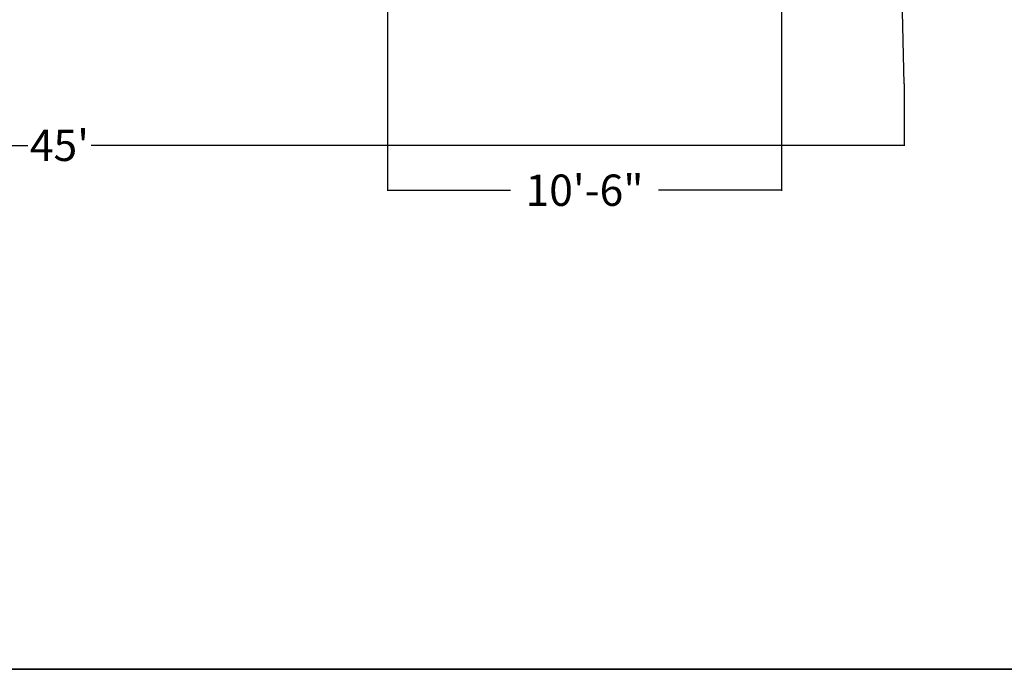
# Model space of a CAD drawing. Units: inches. Extents: x -269 to 4574, y -694 to 313.
# Tile 2 of 19: x 208 to 522, y -694 to -486. Entities that reach past the tile are written whole.
import ezdxf

# ---------------------------------------------------------------- set-up
doc = ezdxf.new("R2010")
doc.units = ezdxf.units.IN
doc.header["$MEASUREMENT"] = 0
for name, color, linetype, lineweight in [('BORDER', 7, 'Continuous', 35), ('C-PROP', 7, 'Continuous', 25), ('DIMENSION', 5, 'Continuous', 18)]:
    doc.layers.add(name, color=color, linetype=linetype, lineweight=lineweight)
doc.dimstyles.get("Standard").update_dxf_attribs({"dimtxt": 10, "dimasz": 0.18, "dimexe": 0.18, "dimexo": 0.0625, "dimgap": 0.09, "dimtad": 0, "dimdec": 1, "dimzin": 0, "dimdsep": 46, "dimlunit": 3, "dimtxsty": 'Standard', "dimcen": 0.09, "dimclrt": 7, "dimadec": 0, "dimazin": 0, "dimtfac": 1, "dimtdec": 1, "dimtofl": 0, "dimtmove": 0, "dimatfit": 3, "dimfxl": 1, "dimtolj": 1, "dimtzin": 0, "dimarcsym": 0})

# ---------------------------------------------------------------- blocks, each defined once
blk = doc.blocks.new('*D33')
at = {"layer": 'Defpoints', "color": 0, "lineweight": 0, "transparency": 16777216}
for p in [(-49.71, -506.83), (490.29, -506.83), (490.29, -526.5)]:
    blk.add_point(p, dxfattribs=at)
at = {"layer": 'DIMENSION', "color": 0, "lineweight": -2, "transparency": 16777216}
for p, q in [((-49.71, -506.9), (-49.71, -526.68)), ((490.29, -506.9), (490.29, -526.68)), ((-49.53, -526.5), (210.2, -526.5)), ((490.11, -526.5), (230.38, -526.5))]:
    blk.add_line(p, q, dxfattribs=at)
at = {"layer": 'DIMENSION', "color": 0, "lineweight": 0, "transparency": 16777216}
for points in [[(-49.53, -526.47), (-49.53, -526.53), (-49.71, -526.5)], [(490.11, -526.47), (490.11, -526.53), (490.29, -526.5)]]:
    blk.add_solid(points, dxfattribs=at)
at = {"layer": 'DIMENSION', "color": 0, "transparency": 16777216, "insert": (220.29, -526.5), "char_height": 10, "attachment_point": 5}
blk.add_mtext("\\A1;45'", dxfattribs=at)
blk = doc.blocks.new('*D84')
at = {"layer": 'Defpoints', "color": 0, "lineweight": 0, "transparency": 16777216}
for p in [(325.14, -443.73), (451.14, -443.73), (325.14, -540.83)]:
    blk.add_point(p, dxfattribs=at)
at = {"layer": 'DIMENSION', "color": 0, "lineweight": -2, "transparency": 16777216}
for p, q in [((325.14, -443.79), (325.14, -541.01)), ((451.14, -443.79), (451.14, -541.01)), ((325.32, -540.83), (364.48, -540.83)), ((450.96, -540.83), (411.8, -540.83))]:
    blk.add_line(p, q, dxfattribs=at)
at = {"layer": 'DIMENSION', "color": 0, "lineweight": 0, "transparency": 16777216}
for points in [[(325.32, -540.8), (325.32, -540.86), (325.14, -540.83)], [(450.96, -540.8), (450.96, -540.86), (451.14, -540.83)]]:
    blk.add_solid(points, dxfattribs=at)
at = {"layer": 'DIMENSION', "color": 7, "transparency": 16777216, "insert": (388.14, -540.83), "char_height": 10, "attachment_point": 5}
blk.add_mtext('\\A1;10\'-6"', dxfattribs=at)

msp = doc.modelspace()

# ---------------------------------------------------------------- linework, layer by layer
at = {"layer": 'BORDER'}
msp.add_lwpolyline([(-268.51, 198.09), (666.62, 198.09), (666.62, -693.82), (-268.51, -693.82)], close=True, dxfattribs=at)
at = {"layer": 'C-PROP'}
msp.add_line((490.29, -506.83), (478.29, 36.26), dxfattribs=at)

# ---------------------------------------------------------------- dimensions: what is measured, and where the dimension line sits
at = {"layer": 'DIMENSION'}
for base, p1, p2, override, picture, middle in [((325.14, -540.83), (451.14, -443.73), (325.14, -443.73), {"dimdec": 1, "dimlfac": 1, "dimrnd": 0, "dimzin": 1, "dimdsep": 46, "dimlunit": 4, "dimfrac": 2}, '*D84', (388.14, -540.83)), ((490.29, -526.5), (-49.71, -506.83), (490.29, -506.83), {"dimclrd": 0, "dimclre": 0, "dimclrt": 0}, '*D33', (220.29, -526.5))]:
    dim = msp.add_linear_dim(base=base, p1=p1, p2=p2, dimstyle='Standard', override=override, dxfattribs=at)
    dim.commit()
    dim.dimension.update_dxf_attribs({"geometry": picture, "text_midpoint": middle})

doc.saveas('drawing.dxf')
